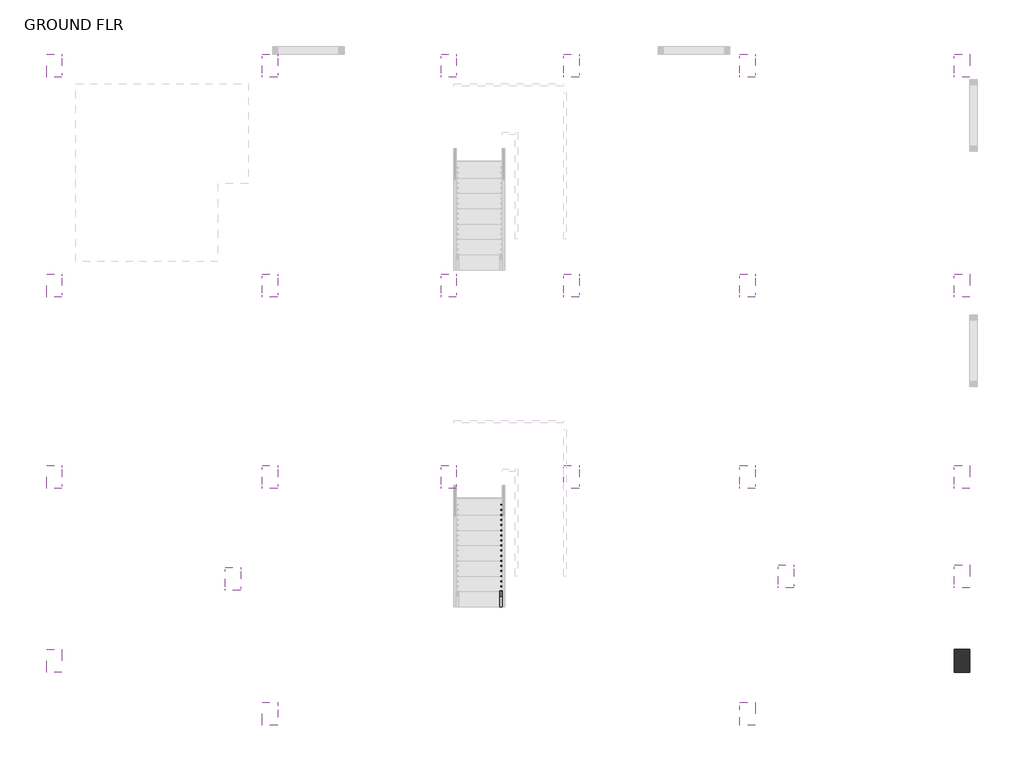
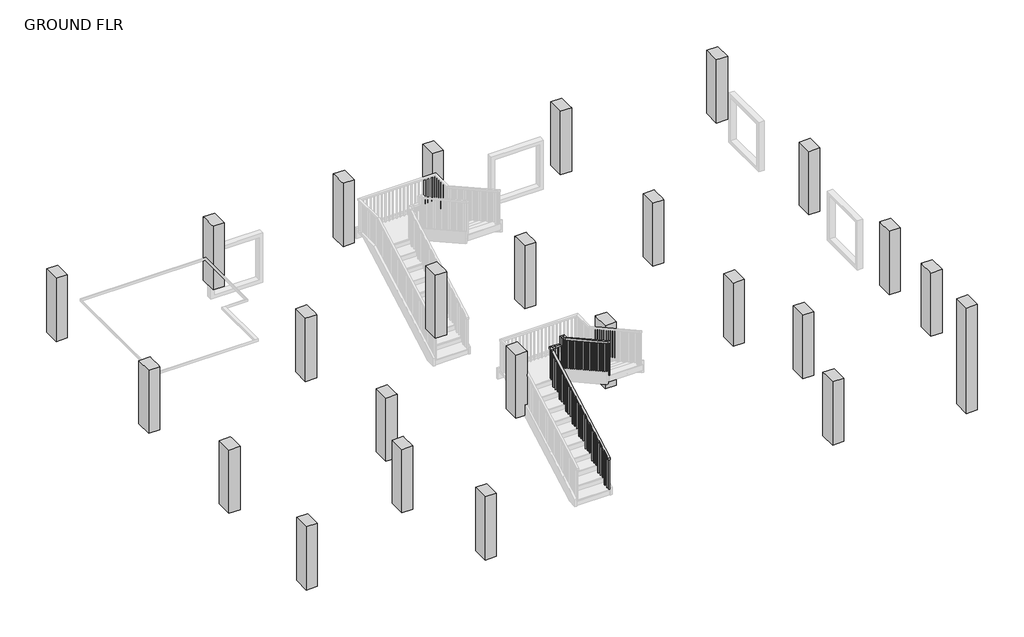
# One storey, part 1 of 4: 25 columns, 1 railing.
"""IFC4 building model written with IfcOpenShell, lengths in millimetres."""

from ifc_helpers import new_model, si_unit, frame, origin, place, context, project, spatial, polyline, outline, extrude, faceted_brep, transform, mapped, element, save
from components import column_6a931455

model = new_model("IFC4")

# Units and contexts
model_context = context("Model", 3, world=origin())
ifc_project = project(units=[si_unit("LENGTHUNIT", "METRE", prefix="MILLI")], contexts=[model_context])

# Site, building, storey
site = spatial("IfcSite", under=ifc_project)
building = spatial("IfcBuilding", under=site)
storey = spatial("IfcBuildingStorey", under=building, Name="GROUND FLR", Elevation=304.8)

# Columns
placement = place(None, origin())
element("IfcColumn", 1, ObjectType="Concrete-Rectangular-Column : 1'6\" X 1' COLUMN", at=placement, inside=storey, context=model_context, shape_type="Brep", body=[
    faceted_brep([(-8839.9786397, -1223.6061634, 1524.0), (-8839.9786397, -1680.8061634, 1524.0), (-9144.7786397, -1680.8061634, 1524.0), (-9144.7786397, -1223.6061634, 1524.0), (-8839.9786397, -1223.6061634, 3352.8), (-8839.9786397, -1299.8061634, 3352.8), (-8839.9786397, -1604.6061634, 3352.8), (-8839.9786397, -1680.8061634, 3352.8), (-8839.9786397, -1680.8061634, 2743.2), (-9144.7786397, -1680.8061634, 3352.8), (-9144.7786397, -1680.8061634, 2743.2), (-9144.7786397, -1223.6061634, 3352.8)], [[[0, 1, 2, 3]], [[4, 5, 6, 7, 8, 1, 0]], [[7, 9, 10, 2, 1, 8]], [[9, 11, 3, 2, 10]], [[11, 4, 0, 3]], [[4, 11, 9, 7, 6, 5]]]),
])
element("IfcColumn", 2, ObjectType="Concrete-Rectangular-Column : 1'6\" X 1' COLUMN", at=placement, inside=storey, context=model_context, shape_type="Brep", body=[
    faceted_brep([(-4548.1175798, -1223.6061634, 1524.0), (-4548.1175798, -1680.8061634, 1524.0), (-4852.9175798, -1680.8061634, 1524.0), (-4852.9175798, -1223.6061634, 1524.0), (-4548.1175798, -1223.6061634, 3352.8), (-4548.1175798, -1299.8061634, 3352.8), (-4548.1175798, -1604.6061634, 3352.8), (-4548.1175798, -1680.8061634, 3352.8), (-4548.1175798, -1680.8061634, 2743.2), (-4852.9175798, -1680.8061634, 3352.8), (-4852.9175798, -1680.8061634, 2743.2), (-4852.9175798, -1604.6061634, 3352.8), (-4852.9175798, -1299.8061634, 3352.8), (-4852.9175798, -1223.6061634, 3352.8)], [[[0, 1, 2, 3]], [[4, 5, 6, 7, 8, 1, 0]], [[7, 9, 10, 2, 1, 8]], [[9, 11, 12, 13, 3, 2, 10]], [[13, 4, 0, 3]], [[4, 13, 12, 11, 9, 7, 6, 5]]]),
])
element("IfcColumn", 3, ObjectType="Concrete-Rectangular-Column : 1'6\" X 1' COLUMN", at=placement, inside=storey, context=model_context, shape_type="Brep", body=[
    faceted_brep([(-992.1175798, -1223.6061634, 1524.0), (-992.1175798, -1680.8061634, 1524.0), (-1296.9175798, -1680.8061634, 1524.0), (-1296.9175798, -1223.6061634, 1524.0), (-992.1175798, -1223.6061634, 3352.8), (-992.1175798, -1299.8061634, 3352.8), (-992.1175798, -1604.6061634, 3352.8), (-992.1175798, -1680.8061634, 3352.8), (-992.1175798, -1680.8061634, 2743.2), (-1296.9175798, -1680.8061634, 3352.8), (-1296.9175798, -1680.8061634, 2743.2), (-1296.9175798, -1604.6061634, 3352.8), (-1296.9175798, -1299.8061634, 3352.8), (-1296.9175798, -1223.6061634, 3352.8)], [[[0, 1, 2, 3]], [[4, 5, 6, 7, 8, 1, 0]], [[7, 9, 10, 2, 1, 8]], [[9, 11, 12, 13, 3, 2, 10]], [[13, 4, 0, 3]], [[4, 13, 12, 11, 9, 7, 6, 5]]]),
])
element("IfcColumn", 4, ObjectType="Concrete-Rectangular-Column : 1'6\" X 1' COLUMN", at=placement, inside=storey, context=model_context, shape_type="Brep", body=[
    faceted_brep([(1446.2824202, -1223.6061634, 1524.0), (1446.2824202, -1680.8061634, 1524.0), (1141.4824202, -1680.8061634, 1524.0), (1141.4824202, -1223.6061634, 1524.0), (1446.2824202, -1223.6061634, 3352.8), (1446.2824202, -1299.8061634, 3352.8), (1446.2824202, -1604.6061634, 3352.8), (1446.2824202, -1680.8061634, 3352.8), (1446.2824202, -1680.8061634, 2743.2), (1141.4824202, -1680.8061634, 3352.8), (1141.4824202, -1680.8061634, 2743.2), (1141.4824202, -1604.6061634, 3352.8), (1141.4824202, -1299.8061634, 3352.8), (1141.4824202, -1223.6061634, 3352.8)], [[[0, 1, 2, 3]], [[4, 5, 6, 7, 8, 1, 0]], [[7, 9, 10, 2, 1, 8]], [[9, 11, 12, 13, 3, 2, 10]], [[13, 4, 0, 3]], [[4, 13, 12, 11, 9, 7, 6, 5]]]),
])
element("IfcColumn", 5, ObjectType="Concrete-Rectangular-Column : 1'6\" X 1' COLUMN", at=placement, inside=storey, context=model_context, shape_type="Brep", body=[
    faceted_brep([(4951.4824202, -1223.6061634, 1524.0), (4951.4824202, -1680.8061634, 1524.0), (4646.6824202, -1680.8061634, 1524.0), (4646.6824202, -1223.6061634, 1524.0), (4951.4824202, -1223.6061634, 3352.8), (4951.4824202, -1299.8061634, 3352.8), (4951.4824202, -1604.6061634, 3352.8), (4951.4824202, -1680.8061634, 3352.8), (4951.4824202, -1680.8061634, 2743.2), (4646.6824202, -1680.8061634, 3352.8), (4646.6824202, -1680.8061634, 2743.2), (4646.6824202, -1604.6061634, 3352.8), (4646.6824202, -1299.8061634, 3352.8), (4646.6824202, -1223.6061634, 3352.8)], [[[0, 1, 2, 3]], [[4, 5, 6, 7, 8, 1, 0]], [[7, 9, 10, 2, 1, 8]], [[9, 11, 12, 13, 3, 2, 10]], [[13, 4, 0, 3]], [[4, 13, 12, 11, 9, 7, 6, 5]]]),
])
element("IfcColumn", 6, ObjectType="Concrete-Rectangular-Column : 1'6\" X 1' COLUMN", at=placement, inside=storey, context=model_context, shape_type="Brep", body=[
    faceted_brep([(9218.6824202, -1223.6061634, 1524.0), (9218.6824202, -1680.8061634, 1524.0), (8913.8824202, -1680.8061634, 1524.0), (8913.8824202, -1223.6061634, 1524.0), (9218.6824202, -1223.6061634, 3352.8), (9218.6824202, -1680.8061634, 3352.8), (9218.6824202, -1680.8061634, 2743.2), (8913.8824202, -1680.8061634, 3352.8), (8913.8824202, -1680.8061634, 2743.2), (8913.8824202, -1604.6061634, 3352.8), (8913.8824202, -1299.8061634, 3352.8), (8913.8824202, -1223.6061634, 3352.8)], [[[0, 1, 2, 3]], [[4, 5, 6, 1, 0]], [[5, 7, 8, 2, 1, 6]], [[7, 9, 10, 11, 3, 2, 8]], [[11, 4, 0, 3]], [[4, 11, 10, 9, 7, 5]]]),
])
element("IfcColumn", 7, ObjectType="Concrete-Rectangular-Column : 1'6\" X 1' COLUMN", at=placement, inside=storey, context=model_context, shape_type="Brep", body=[
    faceted_brep([(9218.6824202, -5600.6620333, 1524.0), (9218.6824202, -6057.8620333, 1524.0), (8913.8824202, -6057.8620333, 1524.0), (8913.8824202, -5600.6620333, 1524.0), (9218.6824202, -5600.6620333, 3352.8), (9218.6824202, -6057.8620333, 3352.8), (9218.6824202, -6057.8620333, 2743.2), (9218.6824202, -5600.6620333, 2743.2), (8913.8824202, -6057.8620333, 3352.8), (8913.8824202, -6057.8620333, 2743.2), (8913.8824202, -5981.6620333, 3352.8), (8913.8824202, -5676.8620333, 3352.8), (8913.8824202, -5600.6620333, 3352.8), (8913.8824202, -5600.6620333, 2743.2)], [[[0, 1, 2, 3]], [[4, 5, 6, 1, 0, 7]], [[5, 8, 9, 2, 1, 6]], [[8, 10, 11, 12, 13, 3, 2, 9]], [[12, 4, 7, 0, 3, 13]], [[4, 12, 11, 10, 8, 5]]]),
])
element("IfcColumn", 8, ObjectType="Concrete-Rectangular-Column : 1'6\" X 1' COLUMN", at=placement, inside=storey, context=model_context, shape_type="Brep", body=[
    faceted_brep([(4951.4824202, -5600.6620333, 1524.0), (4951.4824202, -6057.8620333, 1524.0), (4646.6824202, -6057.8620333, 1524.0), (4646.6824202, -5600.6620333, 1524.0), (4951.4824202, -5600.6620333, 3352.8), (4951.4824202, -5676.8620333, 3352.8), (4951.4824202, -5981.6620333, 3352.8), (4951.4824202, -6057.8620333, 3352.8), (4951.4824202, -6057.8620333, 2743.2), (4951.4824202, -5600.6620333, 2743.2), (4646.6824202, -6057.8620333, 3352.8), (4646.6824202, -6057.8620333, 2743.2), (4646.6824202, -5981.6620333, 3352.8), (4646.6824202, -5676.8620333, 3352.8), (4646.6824202, -5600.6620333, 3352.8), (4646.6824202, -5600.6620333, 2743.2)], [[[0, 1, 2, 3]], [[4, 5, 6, 7, 8, 1, 0, 9]], [[7, 10, 11, 2, 1, 8]], [[10, 12, 13, 14, 15, 3, 2, 11]], [[14, 4, 9, 0, 3, 15]], [[4, 14, 13, 12, 10, 7, 6, 5]]]),
])
element("IfcColumn", 9, ObjectType="Concrete-Rectangular-Column : 1'6\" X 1' COLUMN", at=placement, inside=storey, context=model_context, shape_type="Brep", body=[
    faceted_brep([(1446.2824202, -5600.6620333, 1524.0), (1446.2824202, -6057.8620333, 1524.0), (1141.4824202, -6057.8620333, 1524.0), (1141.4824202, -5600.6620333, 1524.0), (1446.2824202, -5600.6620333, 3352.8), (1446.2824202, -5676.8620333, 3352.8), (1446.2824202, -5981.6620333, 3352.8), (1446.2824202, -6057.8620333, 3352.8), (1446.2824202, -6057.8620333, 2743.2), (1446.2824202, -5600.6620333, 2743.2), (1141.4824202, -6057.8620333, 3352.8), (1141.4824202, -6057.8620333, 2743.2), (1141.4824202, -5981.6620333, 3352.8), (1141.4824202, -5676.8620333, 3352.8), (1141.4824202, -5600.6620333, 3352.8), (1141.4824202, -5600.6620333, 2743.2)], [[[0, 1, 2, 3]], [[4, 5, 6, 7, 8, 1, 0, 9]], [[7, 10, 11, 2, 1, 8]], [[10, 12, 13, 14, 15, 3, 2, 11]], [[14, 4, 9, 0, 3, 15]], [[4, 14, 13, 12, 10, 7, 6, 5]]]),
])
element("IfcColumn", 10, ObjectType="Concrete-Rectangular-Column : 1'6\" X 1' COLUMN", at=placement, inside=storey, context=model_context, shape_type="Brep", body=[
    faceted_brep([(-992.1175798, -5600.6620333, 1524.0), (-992.1175798, -6057.8620333, 1524.0), (-1296.9175798, -6057.8620333, 1524.0), (-1296.9175798, -5600.6620333, 1524.0), (-992.1175798, -5600.6620333, 3352.8), (-992.1175798, -5676.8620333, 3352.8), (-992.1175798, -5981.6620333, 3352.8), (-992.1175798, -6057.8620333, 3352.8), (-992.1175798, -6057.8620333, 2743.2), (-992.1175798, -5600.6620333, 2743.2), (-1296.9175798, -6057.8620333, 3352.8), (-1296.9175798, -6057.8620333, 2743.2), (-1296.9175798, -5981.6620333, 3352.8), (-1296.9175798, -5676.8620333, 3352.8), (-1296.9175798, -5600.6620333, 3352.8), (-1296.9175798, -5600.6620333, 2743.2)], [[[0, 1, 2, 3]], [[4, 5, 6, 7, 8, 1, 0, 9]], [[7, 10, 11, 2, 1, 8]], [[10, 12, 13, 14, 15, 3, 2, 11]], [[14, 4, 9, 0, 3, 15]], [[4, 14, 13, 12, 10, 7, 6, 5]]]),
])
element("IfcColumn", 11, ObjectType="Concrete-Rectangular-Column : 1'6\" X 1' COLUMN", at=placement, inside=storey, context=model_context, shape_type="Brep", body=[
    faceted_brep([(-4548.1175798, -5600.6620333, 1524.0), (-4548.1175798, -6057.8620333, 1524.0), (-4852.9175798, -6057.8620333, 1524.0), (-4852.9175798, -5600.6620333, 1524.0), (-4548.1175798, -5600.6620333, 3352.8), (-4548.1175798, -5676.8620333, 3352.8), (-4548.1175798, -5981.6620333, 3352.8), (-4548.1175798, -6057.8620333, 3352.8), (-4548.1175798, -6057.8620333, 2743.2), (-4548.1175798, -5600.6620333, 2743.2), (-4852.9175798, -6057.8620333, 3352.8), (-4852.9175798, -6057.8620333, 2743.2), (-4852.9175798, -5981.6620333, 3352.8), (-4852.9175798, -5676.8620333, 3352.8), (-4852.9175798, -5600.6620333, 3352.8), (-4852.9175798, -5600.6620333, 2743.2)], [[[0, 1, 2, 3]], [[4, 5, 6, 7, 8, 1, 0, 9]], [[7, 10, 11, 2, 1, 8]], [[10, 12, 13, 14, 15, 3, 2, 11]], [[14, 4, 9, 0, 3, 15]], [[4, 14, 13, 12, 10, 7, 6, 5]]]),
])
element("IfcColumn", 12, ObjectType="Concrete-Rectangular-Column : 1'6\" X 1' COLUMN", at=placement, inside=storey, context=model_context, shape_type="Brep", body=[
    faceted_brep([(-8839.9786397, -5600.6620333, 1524.0), (-8839.9786397, -6057.8620333, 1524.0), (-9144.7786397, -6057.8620333, 1524.0), (-9144.7786397, -5600.6620333, 1524.0), (-8839.9786397, -5600.6620333, 3352.8), (-8839.9786397, -5676.8620333, 3352.8), (-8839.9786397, -5981.6620333, 3352.8), (-8839.9786397, -6057.8620333, 3352.8), (-8839.9786397, -6057.8620333, 2743.2), (-8839.9786397, -5600.6620333, 2743.2), (-9144.7786397, -6057.8620333, 3352.8), (-9144.7786397, -6057.8620333, 2743.2), (-9144.7786397, -5600.6620333, 3352.8), (-9144.7786397, -5600.6620333, 2743.2)], [[[0, 1, 2, 3]], [[4, 5, 6, 7, 8, 1, 0, 9]], [[7, 10, 11, 2, 1, 8]], [[10, 12, 13, 3, 2, 11]], [[12, 4, 9, 0, 3, 13]], [[4, 12, 10, 7, 6, 5]]]),
])
element("IfcColumn", 13, ObjectType="Concrete-Rectangular-Column : 1'6\" X 1' COLUMN", at=placement, inside=storey, context=model_context, shape_type="Brep", body=[
    faceted_brep([(-8839.9786397, -9410.6620333, 1524.0), (-8839.9786397, -9867.8620333, 1524.0), (-9144.7786397, -9867.8620333, 1524.0), (-9144.7786397, -9410.6620333, 1524.0), (-8839.9786397, -9410.6620333, 3352.8), (-8839.9786397, -9486.8620333, 3352.8), (-8839.9786397, -9791.6620333, 3352.8), (-8839.9786397, -9867.8620333, 3352.8), (-8839.9786397, -9867.8620333, 2743.2), (-8839.9786397, -9410.6620333, 2743.2), (-9144.7786397, -9867.8620333, 3352.8), (-9144.7786397, -9867.8620333, 2743.2), (-9144.7786397, -9410.6620333, 3352.8), (-9144.7786397, -9410.6620333, 2743.2)], [[[0, 1, 2, 3]], [[4, 5, 6, 7, 8, 1, 0, 9]], [[7, 10, 11, 2, 1, 8]], [[10, 12, 13, 3, 2, 11]], [[12, 4, 9, 0, 3, 13]], [[4, 12, 10, 7, 6, 5]]]),
])
element("IfcColumn", 14, ObjectType="Concrete-Rectangular-Column : 1'6\" X 1' COLUMN", at=placement, inside=storey, context=model_context, shape_type="Brep", body=[
    faceted_brep([(-4548.1175798, -9410.6620333, 1524.0), (-4548.1175798, -9867.8620333, 1524.0), (-4852.9175798, -9867.8620333, 1524.0), (-4852.9175798, -9410.6620333, 1524.0), (-4548.1175798, -9410.6620333, 3352.8), (-4548.1175798, -9486.8620333, 3352.8), (-4548.1175798, -9791.6620333, 3352.8), (-4548.1175798, -9867.8620333, 3352.8), (-4548.1175798, -9867.8620333, 2743.2), (-4548.1175798, -9410.6620333, 2743.2), (-4852.9175798, -9867.8620333, 3352.8), (-4852.9175798, -9867.8620333, 2743.2), (-4852.9175798, -9791.6620333, 3352.8), (-4852.9175798, -9486.8620333, 3352.8), (-4852.9175798, -9410.6620333, 3352.8), (-4852.9175798, -9410.6620333, 2743.2)], [[[0, 1, 2, 3]], [[4, 5, 6, 7, 8, 1, 0, 9]], [[7, 10, 11, 2, 1, 8]], [[10, 12, 13, 14, 15, 3, 2, 11]], [[14, 4, 9, 0, 3, 15]], [[4, 14, 13, 12, 10, 7, 6, 5]]]),
])
element("IfcColumn", 15, ObjectType="Concrete-Rectangular-Column : 1'6\" X 1' COLUMN", at=placement, inside=storey, context=model_context, shape_type="Brep", body=[
    faceted_brep([(-992.1175798, -9410.6620333, 1524.0), (-992.1175798, -9867.8620333, 1524.0), (-1296.9175798, -9867.8620333, 1524.0), (-1296.9175798, -9410.6620333, 1524.0), (-992.1175798, -9410.6620333, 3352.8), (-992.1175798, -9486.8620333, 3352.8), (-992.1175798, -9791.6620333, 3352.8), (-992.1175798, -9867.8620333, 3352.8), (-992.1175798, -9410.6620333, 2743.2), (-1296.9175798, -9867.8620333, 3352.8), (-1296.9175798, -9791.6620333, 3352.8), (-1296.9175798, -9486.8620333, 3352.8), (-1296.9175798, -9410.6620333, 3352.8), (-1296.9175798, -9410.6620333, 2743.2)], [[[0, 1, 2, 3]], [[4, 5, 6, 7, 1, 0, 8]], [[7, 9, 2, 1]], [[9, 10, 11, 12, 13, 3, 2]], [[12, 4, 8, 0, 3, 13]], [[4, 12, 11, 10, 9, 7, 6, 5]]]),
])
element("IfcColumn", 16, ObjectType="Concrete-Rectangular-Column : 1'6\" X 1' COLUMN", at=placement, inside=storey, context=model_context, shape_type="Brep", body=[
    faceted_brep([(9218.6824202, -11391.8620333, 1524.0), (9218.6824202, -11849.0620333, 1524.0), (8913.8824202, -11849.0620333, 1524.0), (8913.8824202, -11391.8620333, 1524.0), (9218.6824202, -11391.8620333, 3352.8), (9218.6824202, -11849.0620333, 3352.8), (9218.6824202, -11391.8620333, 2743.2), (8913.8824202, -11849.0620333, 3352.8), (8913.8824202, -11772.8620333, 3352.8), (8913.8824202, -11468.0620333, 3352.8), (8913.8824202, -11391.8620333, 3352.8), (8913.8824202, -11391.8620333, 2743.2)], [[[0, 1, 2, 3]], [[4, 5, 1, 0, 6]], [[5, 7, 2, 1]], [[7, 8, 9, 10, 11, 3, 2]], [[10, 4, 6, 0, 3, 11]], [[4, 10, 9, 8, 7, 5]]]),
])
element("IfcColumn", 17, ObjectType="Concrete-Rectangular-Column : 1'6\" X 1' COLUMN", at=placement, inside=storey, context=model_context, shape_type="Brep", body=[
    faceted_brep([(9218.6824202, -9410.6620333, 1524.0), (9218.6824202, -9867.8620333, 1524.0), (8913.8824202, -9867.8620333, 1524.0), (8913.8824202, -9410.6620333, 1524.0), (9218.6824202, -9410.6620333, 3352.8), (9218.6824202, -9867.8620333, 3352.8), (9218.6824202, -9867.8620333, 2743.2), (9218.6824202, -9410.6620333, 2743.2), (8913.8824202, -9867.8620333, 3352.8), (8913.8824202, -9867.8620333, 2743.2), (8913.8824202, -9791.6620333, 3352.8), (8913.8824202, -9486.8620333, 3352.8), (8913.8824202, -9410.6620333, 3352.8), (8913.8824202, -9410.6620333, 2743.2)], [[[0, 1, 2, 3]], [[4, 5, 6, 1, 0, 7]], [[5, 8, 9, 2, 1, 6]], [[8, 10, 11, 12, 13, 3, 2, 9]], [[12, 4, 7, 0, 3, 13]], [[4, 12, 11, 10, 8, 5]]]),
])
element("IfcColumn", 18, ObjectType="Concrete-Rectangular-Column : 1'6\" X 1' COLUMN", at=placement, inside=storey, context=model_context, shape_type="Brep", body=[
    faceted_brep([(4951.4824202, -9410.6620333, 1524.0), (4951.4824202, -9867.8620333, 1524.0), (4646.6824202, -9867.8620333, 1524.0), (4646.6824202, -9410.6620333, 1524.0), (4951.4824202, -9410.6620333, 3352.8), (4951.4824202, -9486.8620333, 3352.8), (4951.4824202, -9791.6620333, 3352.8), (4951.4824202, -9867.8620333, 3352.8), (4951.4824202, -9867.8620333, 2743.2), (4951.4824202, -9410.6620333, 2743.2), (4646.6824202, -9867.8620333, 3352.8), (4646.6824202, -9867.8620333, 2743.2), (4646.6824202, -9791.6620333, 3352.8), (4646.6824202, -9486.8620333, 3352.8), (4646.6824202, -9410.6620333, 3352.8), (4646.6824202, -9410.6620333, 2743.2)], [[[0, 1, 2, 3]], [[4, 5, 6, 7, 8, 1, 0, 9]], [[7, 10, 11, 2, 1, 8]], [[10, 12, 13, 14, 15, 3, 2, 11]], [[14, 4, 9, 0, 3, 15]], [[4, 14, 13, 12, 10, 7, 6, 5]]]),
])
element("IfcColumn", 19, ObjectType="Concrete-Rectangular-Column : 1'6\" X 1' COLUMN", at=placement, inside=storey, context=model_context, shape_type="Brep", body=[
    faceted_brep([(1446.2824202, -9410.6620333, 1524.0), (1446.2824202, -9867.8620333, 1524.0), (1141.4824202, -9867.8620333, 1524.0), (1141.4824202, -9410.6620333, 1524.0), (1446.2824202, -9410.6620333, 3352.8), (1446.2824202, -9486.8620333, 3352.8), (1446.2824202, -9791.6620333, 3352.8), (1446.2824202, -9867.8620333, 3352.8), (1446.2824202, -9410.6620333, 2743.2), (1141.4824202, -9867.8620333, 3352.8), (1141.4824202, -9791.6620333, 3352.8), (1141.4824202, -9486.8620333, 3352.8), (1141.4824202, -9410.6620333, 3352.8), (1141.4824202, -9410.6620333, 2743.2)], [[[0, 1, 2, 3]], [[4, 5, 6, 7, 1, 0, 8]], [[7, 9, 2, 1]], [[9, 10, 11, 12, 13, 3, 2]], [[12, 4, 8, 0, 3, 13]], [[4, 12, 11, 10, 9, 7, 6, 5]]]),
])
element("IfcColumn", 20, ObjectType="Concrete-Rectangular-Column : 1'6\" X 1' COLUMN", at=placement, inside=storey, context=model_context, shape_type="Brep", body=[
    faceted_brep([(-4548.1175798, -14119.6402089, 1524.0), (-4548.1175798, -14576.8402089, 1524.0), (-4852.9175798, -14576.8402089, 1524.0), (-4852.9175798, -14119.6402089, 1524.0), (-4548.1175798, -14119.6402089, 3352.8), (-4548.1175798, -14272.0402089, 3352.8), (-4548.1175798, -14576.8402089, 3352.8), (-4548.1175798, -14576.8402089, 2743.2), (-4548.1175798, -14119.6402089, 2743.2), (-4852.9175798, -14576.8402089, 3352.8), (-4852.9175798, -14119.6402089, 3352.8), (-4852.9175798, -14119.6402089, 2743.2)], [[[0, 1, 2, 3]], [[4, 5, 6, 7, 1, 0, 8]], [[6, 9, 2, 1, 7]], [[9, 10, 11, 3, 2]], [[10, 4, 8, 0, 3, 11]], [[4, 10, 9, 6, 5]]]),
])
element("IfcColumn", 21, ObjectType="Concrete-Rectangular-Column : 1'6\" X 1' COLUMN", at=placement, inside=storey, context=model_context, shape_type="Brep", body=[
    faceted_brep([(-8839.9786397, -13068.2620333, 1524.0), (-8839.9786397, -13525.4620333, 1524.0), (-9144.7786397, -13525.4620333, 1524.0), (-9144.7786397, -13068.2620333, 1524.0), (-8839.9786397, -13068.2620333, 3352.8), (-8839.9786397, -13525.4620333, 3352.8), (-8839.9786397, -13068.2620333, 2743.2), (-9144.7786397, -13525.4620333, 3352.8), (-9144.7786397, -13068.2620333, 3352.8), (-9144.7786397, -13068.2620333, 2743.2)], [[[0, 1, 2, 3]], [[4, 5, 1, 0, 6]], [[5, 7, 2, 1]], [[7, 8, 9, 3, 2]], [[8, 4, 6, 0, 3, 9]], [[4, 8, 7, 5]]]),
])
element("IfcColumn", 22, ObjectType="Concrete-Rectangular-Column : 1'6\" X 1' COLUMN", at=placement, inside=storey, context=model_context, shape_type="Brep", body=[
    faceted_brep([(-5284.7175798, -11442.6620333, 1524.0), (-5284.7175798, -11899.8620333, 1524.0), (-5589.5175798, -11899.8620333, 1524.0), (-5589.5175798, -11442.6620333, 1524.0), (-5284.7175798, -11442.6620333, 3352.8), (-5284.7175798, -11518.8620333, 3352.8), (-5284.7175798, -11823.6620333, 3352.8), (-5284.7175798, -11899.8620333, 3352.8), (-5589.5175798, -11899.8620333, 3352.8), (-5589.5175798, -11823.6620333, 3352.8), (-5589.5175798, -11518.8620333, 3352.8), (-5589.5175798, -11442.6620333, 3352.8)], [[[0, 1, 2, 3]], [[4, 5, 6, 7, 1, 0]], [[7, 8, 2, 1]], [[8, 9, 10, 11, 3, 2]], [[11, 4, 0, 3]], [[4, 11, 10, 9, 8, 7, 6, 5]]]),
])
element("IfcColumn", 23, ObjectType="Concrete-Rectangular-Column : 1'6\" X 1' COLUMN", at=placement, inside=storey, context=model_context, shape_type="Brep", body=[
    faceted_brep([(5713.4824202, -11391.8620333, 1524.0), (5713.4824202, -11849.0620333, 1524.0), (5408.6824202, -11849.0620333, 1524.0), (5408.6824202, -11391.8620333, 1524.0), (5713.4824202, -11391.8620333, 3352.8), (5713.4824202, -11468.0620333, 3352.8), (5713.4824202, -11772.8620333, 3352.8), (5713.4824202, -11849.0620333, 3352.8), (5408.6824202, -11849.0620333, 3352.8), (5408.6824202, -11772.8620333, 3352.8), (5408.6824202, -11468.0620333, 3352.8), (5408.6824202, -11391.8620333, 3352.8)], [[[0, 1, 2, 3]], [[4, 5, 6, 7, 1, 0]], [[7, 8, 2, 1]], [[8, 9, 10, 11, 3, 2]], [[11, 4, 0, 3]], [[4, 11, 10, 9, 8, 7, 6, 5]]]),
])
element("IfcColumn", 24, ObjectType="Concrete-Rectangular-Column : 1'6\" X 1' COLUMN", at=placement, inside=storey, context=model_context, shape_type="Brep", body=[
    faceted_brep([(4951.4824202, -14119.6402089, 1524.0), (4951.4824202, -14576.8402089, 1524.0), (4646.6824202, -14576.8402089, 1524.0), (4646.6824202, -14119.6402089, 1524.0), (4951.4824202, -14119.6402089, 3352.8), (4951.4824202, -14576.8402089, 3352.8), (4951.4824202, -14119.6402089, 2743.2), (4646.6824202, -14576.8402089, 3352.8), (4646.6824202, -14576.8402089, 2743.2), (4646.6824202, -14272.0402089, 3352.8), (4646.6824202, -14119.6402089, 3352.8), (4646.6824202, -14119.6402089, 2743.2)], [[[0, 1, 2, 3]], [[4, 5, 1, 0, 6]], [[5, 7, 8, 2, 1]], [[7, 9, 10, 11, 3, 2, 8]], [[10, 4, 6, 0, 3, 11]], [[4, 10, 9, 7, 5]]]),
])
column_shape = column_6a931455(model_context)
element("IfcColumn", 25, ObjectType="Concrete-Rectangular-Column : 1'6\" X 1' COLUMN", at=placement, inside=storey, context=model_context, shape_type="MappedRepresentation", body=[
    mapped(column_shape, transform((9066.2824202, -13294.1402089, 0.0), x_axis=(1.0, 0.0, 0.0), y_axis=(0.0, 1.0, 0.0), z_axis=(0.0, 0.0, 1.0))),
])

# Railing
element("IfcRailing", 26, ObjectType="Handrail - Rectangular", at=placement, inside=storey, context=model_context, shape_type="SolidModel", body=[
    faceted_brep([(-128.5175798, -12221.8061634, 1388.5333333), (-128.5175798, -12221.8061634, 1330.420221), (-77.7175798, -12221.8061634, 1330.420221), (-77.7175798, -12221.8061634, 1388.5333333), (-128.5175798, -9554.8061634, 2870.2), (-128.5175798, -9504.0061634, 2840.3091099), (-77.7175798, -9504.0061634, 2840.3091099), (-77.7175798, -9554.8061634, 2870.2), (-128.5175798, -9554.8061634, 2912.5333333), (-128.5175798, -9504.0061634, 2861.7333333), (-77.7175798, -9504.0061634, 2861.7333333), (-77.7175798, -9554.8061634, 2912.5333333), (-128.5175798, -9427.8061634, 2912.5333333), (-128.5175798, -9427.8061634, 2861.7333333), (-77.7175798, -9478.6061634, 2861.7333333), (-77.7175798, -9478.6061634, 2912.5333333), (-1.5175798, -9427.8061634, 2912.5333333), (-1.5175798, -9427.8061634, 2861.7333333), (-1.5175798, -9478.6061634, 2861.7333333), (-1.5175798, -9478.6061634, 2912.5333333), (150.8824202, -9427.8061634, 2912.5333333), (201.6824202, -9427.8061634, 2861.7333333), (201.6824202, -9478.6061634, 2861.7333333), (150.8824202, -9478.6061634, 2912.5333333), (150.8824202, -9427.8061634, 3124.2), (201.6824202, -9427.8061634, 3073.4), (201.6824202, -9478.6061634, 3073.4), (150.8824202, -9478.6061634, 3124.2), (277.8824202, -9427.8061634, 3124.2), (277.8824202, -9427.8061634, 3073.4), (227.0824202, -9478.6061634, 3073.4), (227.0824202, -9478.6061634, 3124.2), (277.8824202, -9554.8061634, 3124.2), (277.8824202, -9567.9697656, 3073.4), (227.0824202, -9567.9697656, 3073.4), (227.0824202, -9554.8061634, 3124.2), (277.8824202, -11612.2061634, 4267.2), (227.0824202, -11612.2061634, 4267.2), (227.0824202, -11612.2061634, 4209.0868876), (277.8824202, -11612.2061634, 4209.0868876)], [[[0, 1, 2, 3]], [[1, 0, 4, 5]], [[2, 1, 5, 6]], [[3, 2, 6, 7]], [[0, 3, 7, 4]], [[5, 4, 8, 9]], [[6, 5, 9, 10]], [[7, 6, 10, 11]], [[4, 7, 11, 8]], [[9, 8, 12, 13]], [[10, 9, 13, 14]], [[11, 10, 14, 15]], [[8, 11, 15, 12]], [[13, 12, 16, 17]], [[14, 13, 17, 18]], [[15, 14, 18, 19]], [[12, 15, 19, 16]], [[17, 16, 20, 21]], [[18, 17, 21, 22]], [[19, 18, 22, 23]], [[16, 19, 23, 20]], [[21, 20, 24, 25]], [[22, 21, 25, 26]], [[23, 22, 26, 27]], [[20, 23, 27, 24]], [[25, 24, 28, 29]], [[26, 25, 29, 30]], [[27, 26, 30, 31]], [[24, 27, 31, 28]], [[29, 28, 32, 33]], [[30, 29, 33, 34]], [[31, 30, 34, 35]], [[28, 31, 35, 32]], [[36, 37, 38, 39]], [[33, 32, 36, 39]], [[34, 33, 39, 38]], [[35, 34, 38, 37]], [[32, 35, 37, 36]]]),
    extrude(outline(polyline([(-11596.3311634, 4200.2674432), (-11577.2811634, 4189.6841099), (-11577.2811634, 3183.4666667), (-11596.3311634, 3183.4666667), (-11596.3311634, 4200.2674432)])), frame((242.9574202, 0.0, 0.0), z_axis=(1.0, 0.0, 0.0), x_axis=(0.0, 1.0, 0.0)), (0.0, 0.0, 1.0), 19.05),
    extrude(outline(polyline([(-11494.7311634, 4143.8229988), (-11475.6811634, 4133.2396654), (-11475.6811634, 3183.4666667), (-11494.7311634, 3183.4666667), (-11494.7311634, 4143.8229988)])), frame((242.9574202, 0.0, 0.0), z_axis=(1.0, 0.0, 0.0), x_axis=(0.0, 1.0, 0.0)), (0.0, 0.0, 1.0), 19.05),
    extrude(outline(polyline([(-11393.1311634, 4087.3785543), (-11374.0811634, 4076.795221), (-11374.0811634, 3183.4666667), (-11393.1311634, 3183.4666667), (-11393.1311634, 4087.3785543)])), frame((242.9574202, 0.0, 0.0), z_axis=(1.0, 0.0, 0.0), x_axis=(0.0, 1.0, 0.0)), (0.0, 0.0, 1.0), 19.05),
    extrude(outline(polyline([(-11291.5311634, 4030.9341099), (-11272.4811634, 4020.3507765), (-11272.4811634, 3014.1333333), (-11291.5311634, 3014.1333333), (-11291.5311634, 4030.9341099)])), frame((242.9574202, 0.0, 0.0), z_axis=(1.0, 0.0, 0.0), x_axis=(0.0, 1.0, 0.0)), (0.0, 0.0, 1.0), 19.05),
    extrude(outline(polyline([(-11189.9311634, 3974.4896654), (-11170.8811634, 3963.9063321), (-11170.8811634, 3014.1333333), (-11189.9311634, 3014.1333333), (-11189.9311634, 3974.4896654)])), frame((242.9574202, 0.0, 0.0), z_axis=(1.0, 0.0, 0.0), x_axis=(0.0, 1.0, 0.0)), (0.0, 0.0, 1.0), 19.05),
    extrude(outline(polyline([(-11088.3311634, 3918.045221), (-11069.2811634, 3907.4618876), (-11069.2811634, 3014.1333333), (-11088.3311634, 3014.1333333), (-11088.3311634, 3918.045221)])), frame((242.9574202, 0.0, 0.0), z_axis=(1.0, 0.0, 0.0), x_axis=(0.0, 1.0, 0.0)), (0.0, 0.0, 1.0), 19.05),
    extrude(outline(polyline([(-10986.7311634, 3861.6007765), (-10967.6811634, 3851.0174432), (-10967.6811634, 2844.8), (-10986.7311634, 2844.8), (-10986.7311634, 3861.6007765)])), frame((242.9574202, 0.0, 0.0), z_axis=(1.0, 0.0, 0.0), x_axis=(0.0, 1.0, 0.0)), (0.0, 0.0, 1.0), 19.05),
    extrude(outline(polyline([(-10885.1311634, 3805.1563321), (-10866.0811634, 3794.5729988), (-10866.0811634, 2844.8), (-10885.1311634, 2844.8), (-10885.1311634, 3805.1563321)])), frame((242.9574202, 0.0, 0.0), z_axis=(1.0, 0.0, 0.0), x_axis=(0.0, 1.0, 0.0)), (0.0, 0.0, 1.0), 19.05),
    extrude(outline(polyline([(-10783.5311634, 3748.7118876), (-10764.4811634, 3738.1285543), (-10764.4811634, 2844.8), (-10783.5311634, 2844.8), (-10783.5311634, 3748.7118876)])), frame((242.9574202, 0.0, 0.0), z_axis=(1.0, 0.0, 0.0), x_axis=(0.0, 1.0, 0.0)), (0.0, 0.0, 1.0), 19.05),
    extrude(outline(polyline([(-10681.9311634, 3692.2674432), (-10662.8811634, 3681.6841099), (-10662.8811634, 2675.4666667), (-10681.9311634, 2675.4666667), (-10681.9311634, 3692.2674432)])), frame((242.9574202, 0.0, 0.0), z_axis=(1.0, 0.0, 0.0), x_axis=(0.0, 1.0, 0.0)), (0.0, 0.0, 1.0), 19.05),
    extrude(outline(polyline([(-10580.3311634, 3635.8229988), (-10561.2811634, 3625.2396654), (-10561.2811634, 2675.4666667), (-10580.3311634, 2675.4666667), (-10580.3311634, 3635.8229988)])), frame((242.9574202, 0.0, 0.0), z_axis=(1.0, 0.0, 0.0), x_axis=(0.0, 1.0, 0.0)), (0.0, 0.0, 1.0), 19.05),
    extrude(outline(polyline([(-10478.7311634, 3579.3785543), (-10459.6811634, 3568.795221), (-10459.6811634, 2675.4666667), (-10478.7311634, 2675.4666667), (-10478.7311634, 3579.3785543)])), frame((242.9574202, 0.0, 0.0), z_axis=(1.0, 0.0, 0.0), x_axis=(0.0, 1.0, 0.0)), (0.0, 0.0, 1.0), 19.05),
    extrude(outline(polyline([(-10377.1311634, 3522.9341099), (-10358.0811634, 3512.3507765), (-10358.0811634, 2506.1333333), (-10377.1311634, 2506.1333333), (-10377.1311634, 3522.9341099)])), frame((242.9574202, 0.0, 0.0), z_axis=(1.0, 0.0, 0.0), x_axis=(0.0, 1.0, 0.0)), (0.0, 0.0, 1.0), 19.05),
    extrude(outline(polyline([(-10275.5311634, 3466.4896654), (-10256.4811634, 3455.9063321), (-10256.4811634, 2506.1333333), (-10275.5311634, 2506.1333333), (-10275.5311634, 3466.4896654)])), frame((242.9574202, 0.0, 0.0), z_axis=(1.0, 0.0, 0.0), x_axis=(0.0, 1.0, 0.0)), (0.0, 0.0, 1.0), 19.05),
    extrude(outline(polyline([(-10173.9311634, 3410.045221), (-10154.8811634, 3399.4618876), (-10154.8811634, 2506.1333333), (-10173.9311634, 2506.1333333), (-10173.9311634, 3410.045221)])), frame((242.9574202, 0.0, 0.0), z_axis=(1.0, 0.0, 0.0), x_axis=(0.0, 1.0, 0.0)), (0.0, 0.0, 1.0), 19.05),
    extrude(outline(polyline([(-10072.3311634, 3353.6007765), (-10053.2811634, 3343.0174432), (-10053.2811634, 2336.8), (-10072.3311634, 2336.8), (-10072.3311634, 3353.6007765)])), frame((242.9574202, 0.0, 0.0), z_axis=(1.0, 0.0, 0.0), x_axis=(0.0, 1.0, 0.0)), (0.0, 0.0, 1.0), 19.05),
    extrude(outline(polyline([(-9970.7311634, 3297.1563321), (-9951.6811634, 3286.5729988), (-9951.6811634, 2336.8), (-9970.7311634, 2336.8), (-9970.7311634, 3297.1563321)])), frame((242.9574202, 0.0, 0.0), z_axis=(1.0, 0.0, 0.0), x_axis=(0.0, 1.0, 0.0)), (0.0, 0.0, 1.0), 19.05),
    extrude(outline(polyline([(-9869.1311634, 3240.7118876), (-9850.0811634, 3230.1285543), (-9850.0811634, 2336.8), (-9869.1311634, 2336.8), (-9869.1311634, 3240.7118876)])), frame((242.9574202, 0.0, 0.0), z_axis=(1.0, 0.0, 0.0), x_axis=(0.0, 1.0, 0.0)), (0.0, 0.0, 1.0), 19.05),
    extrude(outline(polyline([(-9767.5311634, 3184.2674432), (-9748.4811634, 3173.6841099), (-9748.4811634, 2167.4666667), (-9767.5311634, 2167.4666667), (-9767.5311634, 3184.2674432)])), frame((242.9574202, 0.0, 0.0), z_axis=(1.0, 0.0, 0.0), x_axis=(0.0, 1.0, 0.0)), (0.0, 0.0, 1.0), 19.05),
    extrude(outline(polyline([(-9665.9311634, 3127.8229988), (-9646.8811634, 3117.2396654), (-9646.8811634, 2167.4666667), (-9665.9311634, 2167.4666667), (-9665.9311634, 3127.8229988)])), frame((242.9574202, 0.0, 0.0), z_axis=(1.0, 0.0, 0.0), x_axis=(0.0, 1.0, 0.0)), (0.0, 0.0, 1.0), 19.05),
    extrude(outline(polyline([(-9564.3311634, 3071.3785543), (-9545.2811634, 3060.795221), (-9545.2811634, 2167.4666667), (-9564.3311634, 2167.4666667), (-9564.3311634, 3071.3785543)])), frame((242.9574202, 0.0, 0.0), z_axis=(1.0, 0.0, 0.0), x_axis=(0.0, 1.0, 0.0)), (0.0, 0.0, 1.0), 19.05),
    extrude(outline(polyline([(192.1574202, -9462.7311634), (192.1574202, -9443.6811634), (211.2074202, -9443.6811634), (211.2074202, -9462.7311634), (192.1574202, -9462.7311634)])), frame((0.0, 0.0, 1998.1333333), z_axis=(0.0, 0.0, 1.0), x_axis=(1.0, 0.0, 0.0)), (0.0, 0.0, 1.0), 1075.2666667),
    extrude(outline(polyline([(90.5574202, -9462.7311634), (90.5574202, -9443.6811634), (109.6074202, -9443.6811634), (109.6074202, -9462.7311634), (90.5574202, -9462.7311634)])), frame((0.0, 0.0, 1998.1333333), z_axis=(0.0, 0.0, 1.0), x_axis=(1.0, 0.0, 0.0)), (0.0, 0.0, 1.0), 863.6),
    extrude(outline(polyline([(-11.0425798, -9462.7311634), (-11.0425798, -9443.6811634), (8.0074202, -9443.6811634), (8.0074202, -9462.7311634), (-11.0425798, -9462.7311634)])), frame((0.0, 0.0, 1998.1333333), z_axis=(0.0, 0.0, 1.0), x_axis=(1.0, 0.0, 0.0)), (0.0, 0.0, 1.0), 863.6),
    extrude(outline(polyline([(-93.5925798, -9488.1311634), (-112.6425798, -9488.1311634), (-112.6425798, -9469.0811634), (-93.5925798, -9469.0811634), (-93.5925798, -9488.1311634)])), frame((0.0, 0.0, 1998.1333333), z_axis=(0.0, 0.0, 1.0), x_axis=(1.0, 0.0, 0.0)), (0.0, 0.0, 1.0), 863.6),
    extrude(outline(polyline([(-9589.7311634, 2792.6841099), (-9570.6811634, 2803.2674432), (-9570.6811634, 1828.8), (-9589.7311634, 1828.8), (-9589.7311634, 2792.6841099)])), frame((-112.6425798, 0.0, 0.0), z_axis=(1.0, 0.0, 0.0), x_axis=(0.0, 1.0, 0.0)), (0.0, 0.0, 1.0), 19.05),
    extrude(outline(polyline([(-9691.3311634, 2736.2396654), (-9672.2811634, 2746.8229988), (-9672.2811634, 1828.8), (-9691.3311634, 1828.8), (-9691.3311634, 2736.2396654)])), frame((-112.6425798, 0.0, 0.0), z_axis=(1.0, 0.0, 0.0), x_axis=(0.0, 1.0, 0.0)), (0.0, 0.0, 1.0), 19.05),
    extrude(outline(polyline([(-9792.9311634, 2679.795221), (-9773.8811634, 2690.3785543), (-9773.8811634, 1828.8), (-9792.9311634, 1828.8), (-9792.9311634, 2679.795221)])), frame((-112.6425798, 0.0, 0.0), z_axis=(1.0, 0.0, 0.0), x_axis=(0.0, 1.0, 0.0)), (0.0, 0.0, 1.0), 19.05),
    extrude(outline(polyline([(-9894.5311634, 2623.3507765), (-9875.4811634, 2633.9341099), (-9875.4811634, 1659.4666667), (-9894.5311634, 1659.4666667), (-9894.5311634, 2623.3507765)])), frame((-112.6425798, 0.0, 0.0), z_axis=(1.0, 0.0, 0.0), x_axis=(0.0, 1.0, 0.0)), (0.0, 0.0, 1.0), 19.05),
    extrude(outline(polyline([(-9996.1311634, 2566.9063321), (-9977.0811634, 2577.4896654), (-9977.0811634, 1659.4666667), (-9996.1311634, 1659.4666667), (-9996.1311634, 2566.9063321)])), frame((-112.6425798, 0.0, 0.0), z_axis=(1.0, 0.0, 0.0), x_axis=(0.0, 1.0, 0.0)), (0.0, 0.0, 1.0), 19.05),
    extrude(outline(polyline([(-10097.7311634, 2510.4618876), (-10078.6811634, 2521.045221), (-10078.6811634, 1659.4666667), (-10097.7311634, 1659.4666667), (-10097.7311634, 2510.4618876)])), frame((-112.6425798, 0.0, 0.0), z_axis=(1.0, 0.0, 0.0), x_axis=(0.0, 1.0, 0.0)), (0.0, 0.0, 1.0), 19.05),
    extrude(outline(polyline([(-10199.3311634, 2454.0174432), (-10180.2811634, 2464.6007765), (-10180.2811634, 1490.1333333), (-10199.3311634, 1490.1333333), (-10199.3311634, 2454.0174432)])), frame((-112.6425798, 0.0, 0.0), z_axis=(1.0, 0.0, 0.0), x_axis=(0.0, 1.0, 0.0)), (0.0, 0.0, 1.0), 19.05),
    extrude(outline(polyline([(-10300.9311634, 2397.5729988), (-10281.8811634, 2408.1563321), (-10281.8811634, 1490.1333333), (-10300.9311634, 1490.1333333), (-10300.9311634, 2397.5729988)])), frame((-112.6425798, 0.0, 0.0), z_axis=(1.0, 0.0, 0.0), x_axis=(0.0, 1.0, 0.0)), (0.0, 0.0, 1.0), 19.05),
    extrude(outline(polyline([(-10402.5311634, 2341.1285543), (-10383.4811634, 2351.7118876), (-10383.4811634, 1490.1333333), (-10402.5311634, 1490.1333333), (-10402.5311634, 2341.1285543)])), frame((-112.6425798, 0.0, 0.0), z_axis=(1.0, 0.0, 0.0), x_axis=(0.0, 1.0, 0.0)), (0.0, 0.0, 1.0), 19.05),
    extrude(outline(polyline([(-10504.1311634, 2284.6841099), (-10485.0811634, 2295.2674432), (-10485.0811634, 1320.8), (-10504.1311634, 1320.8), (-10504.1311634, 2284.6841099)])), frame((-112.6425798, 0.0, 0.0), z_axis=(1.0, 0.0, 0.0), x_axis=(0.0, 1.0, 0.0)), (0.0, 0.0, 1.0), 19.05),
    extrude(outline(polyline([(-10605.7311634, 2228.2396654), (-10586.6811634, 2238.8229988), (-10586.6811634, 1320.8), (-10605.7311634, 1320.8), (-10605.7311634, 2228.2396654)])), frame((-112.6425798, 0.0, 0.0), z_axis=(1.0, 0.0, 0.0), x_axis=(0.0, 1.0, 0.0)), (0.0, 0.0, 1.0), 19.05),
    extrude(outline(polyline([(-10707.3311634, 2171.795221), (-10688.2811634, 2182.3785543), (-10688.2811634, 1320.8), (-10707.3311634, 1320.8), (-10707.3311634, 2171.795221)])), frame((-112.6425798, 0.0, 0.0), z_axis=(1.0, 0.0, 0.0), x_axis=(0.0, 1.0, 0.0)), (0.0, 0.0, 1.0), 19.05),
    extrude(outline(polyline([(-10808.9311634, 2115.3507765), (-10789.8811634, 2125.9341099), (-10789.8811634, 1151.4666667), (-10808.9311634, 1151.4666667), (-10808.9311634, 2115.3507765)])), frame((-112.6425798, 0.0, 0.0), z_axis=(1.0, 0.0, 0.0), x_axis=(0.0, 1.0, 0.0)), (0.0, 0.0, 1.0), 19.05),
    extrude(outline(polyline([(-10910.5311634, 2058.9063321), (-10891.4811634, 2069.4896654), (-10891.4811634, 1151.4666667), (-10910.5311634, 1151.4666667), (-10910.5311634, 2058.9063321)])), frame((-112.6425798, 0.0, 0.0), z_axis=(1.0, 0.0, 0.0), x_axis=(0.0, 1.0, 0.0)), (0.0, 0.0, 1.0), 19.05),
    extrude(outline(polyline([(-11012.1311634, 2002.4618876), (-10993.0811634, 2013.045221), (-10993.0811634, 1151.4666667), (-11012.1311634, 1151.4666667), (-11012.1311634, 2002.4618876)])), frame((-112.6425798, 0.0, 0.0), z_axis=(1.0, 0.0, 0.0), x_axis=(0.0, 1.0, 0.0)), (0.0, 0.0, 1.0), 19.05),
    extrude(outline(polyline([(-11113.7311634, 1946.0174432), (-11094.6811634, 1956.6007765), (-11094.6811634, 982.1333333), (-11113.7311634, 982.1333333), (-11113.7311634, 1946.0174432)])), frame((-112.6425798, 0.0, 0.0), z_axis=(1.0, 0.0, 0.0), x_axis=(0.0, 1.0, 0.0)), (0.0, 0.0, 1.0), 19.05),
    extrude(outline(polyline([(-11215.3311634, 1889.5729988), (-11196.2811634, 1900.1563321), (-11196.2811634, 982.1333333), (-11215.3311634, 982.1333333), (-11215.3311634, 1889.5729988)])), frame((-112.6425798, 0.0, 0.0), z_axis=(1.0, 0.0, 0.0), x_axis=(0.0, 1.0, 0.0)), (0.0, 0.0, 1.0), 19.05),
    extrude(outline(polyline([(-11316.9311634, 1833.1285543), (-11297.8811634, 1843.7118876), (-11297.8811634, 982.1333333), (-11316.9311634, 982.1333333), (-11316.9311634, 1833.1285543)])), frame((-112.6425798, 0.0, 0.0), z_axis=(1.0, 0.0, 0.0), x_axis=(0.0, 1.0, 0.0)), (0.0, 0.0, 1.0), 19.05),
    extrude(outline(polyline([(-11418.5311634, 1776.6841099), (-11399.4811634, 1787.2674432), (-11399.4811634, 812.8), (-11418.5311634, 812.8), (-11418.5311634, 1776.6841099)])), frame((-112.6425798, 0.0, 0.0), z_axis=(1.0, 0.0, 0.0), x_axis=(0.0, 1.0, 0.0)), (0.0, 0.0, 1.0), 19.05),
    extrude(outline(polyline([(-11520.1311634, 1720.2396654), (-11501.0811634, 1730.8229988), (-11501.0811634, 812.8), (-11520.1311634, 812.8), (-11520.1311634, 1720.2396654)])), frame((-112.6425798, 0.0, 0.0), z_axis=(1.0, 0.0, 0.0), x_axis=(0.0, 1.0, 0.0)), (0.0, 0.0, 1.0), 19.05),
    extrude(outline(polyline([(-11621.7311634, 1663.795221), (-11602.6811634, 1674.3785543), (-11602.6811634, 812.8), (-11621.7311634, 812.8), (-11621.7311634, 1663.795221)])), frame((-112.6425798, 0.0, 0.0), z_axis=(1.0, 0.0, 0.0), x_axis=(0.0, 1.0, 0.0)), (0.0, 0.0, 1.0), 19.05),
    extrude(outline(polyline([(-11723.3311634, 1607.3507765), (-11704.2811634, 1617.9341099), (-11704.2811634, 643.4666667), (-11723.3311634, 643.4666667), (-11723.3311634, 1607.3507765)])), frame((-112.6425798, 0.0, 0.0), z_axis=(1.0, 0.0, 0.0), x_axis=(0.0, 1.0, 0.0)), (0.0, 0.0, 1.0), 19.05),
    extrude(outline(polyline([(-11824.9311634, 1550.9063321), (-11805.8811634, 1561.4896654), (-11805.8811634, 643.4666667), (-11824.9311634, 643.4666667), (-11824.9311634, 1550.9063321)])), frame((-112.6425798, 0.0, 0.0), z_axis=(1.0, 0.0, 0.0), x_axis=(0.0, 1.0, 0.0)), (0.0, 0.0, 1.0), 19.05),
    extrude(outline(polyline([(-11926.5311634, 1494.4618876), (-11907.4811634, 1505.045221), (-11907.4811634, 643.4666667), (-11926.5311634, 643.4666667), (-11926.5311634, 1494.4618876)])), frame((-112.6425798, 0.0, 0.0), z_axis=(1.0, 0.0, 0.0), x_axis=(0.0, 1.0, 0.0)), (0.0, 0.0, 1.0), 19.05),
    extrude(outline(polyline([(-12028.1311634, 1438.0174432), (-12009.0811634, 1448.6007765), (-12009.0811634, 474.1333333), (-12028.1311634, 474.1333333), (-12028.1311634, 1438.0174432)])), frame((-112.6425798, 0.0, 0.0), z_axis=(1.0, 0.0, 0.0), x_axis=(0.0, 1.0, 0.0)), (0.0, 0.0, 1.0), 19.05),
    extrude(outline(polyline([(-12129.7311634, 1381.5729988), (-12110.6811634, 1392.1563321), (-12110.6811634, 474.1333333), (-12129.7311634, 474.1333333), (-12129.7311634, 1381.5729988)])), frame((-112.6425798, 0.0, 0.0), z_axis=(1.0, 0.0, 0.0), x_axis=(0.0, 1.0, 0.0)), (0.0, 0.0, 1.0), 19.05),
    extrude(outline(polyline([(242.9574202, -9462.7311634), (242.9574202, -9443.6811634), (262.0074202, -9443.6811634), (262.0074202, -9462.7311634), (242.9574202, -9462.7311634)])), frame((0.0, 0.0, 1998.1333333), z_axis=(0.0, 0.0, 1.0), x_axis=(1.0, 0.0, 0.0)), (0.0, 0.0, 1.0), 1075.2666667),
    extrude(outline(polyline([(-93.5925798, -9462.7311634), (-112.6425798, -9462.7311634), (-112.6425798, -9443.6811634), (-93.5925798, -9443.6811634), (-93.5925798, -9462.7311634)])), frame((0.0, 0.0, 1998.1333333), z_axis=(0.0, 0.0, 1.0), x_axis=(1.0, 0.0, 0.0)), (0.0, 0.0, 1.0), 863.6),
    extrude(outline(polyline([(-11612.2061634, 4209.0868876), (-11593.1561634, 4198.5035543), (-11593.1561634, 3183.4666667), (-11612.2061634, 3183.4666667), (-11612.2061634, 4209.0868876)])), frame((242.9574202, 0.0, 0.0), z_axis=(1.0, 0.0, 0.0), x_axis=(0.0, 1.0, 0.0)), (0.0, 0.0, 1.0), 19.05),
    extrude(outline(polyline([(-12221.8061634, 1330.420221), (-12202.7561634, 1341.0035543), (-12202.7561634, 474.1333333), (-12221.8061634, 474.1333333), (-12221.8061634, 1330.420221)])), frame((-112.6425798, 0.0, 0.0), z_axis=(1.0, 0.0, 0.0), x_axis=(0.0, 1.0, 0.0)), (0.0, 0.0, 1.0), 19.05),
])

save(model, "model.ifc")

# Revit data of these elements
# Type "Concrete-Rectangular-Column : 1'6\" X 1' COLUMN"
#   Assembly Code = "B10"
#   b = 1' - 0"
#   h = 1' - 6"
#   Structural Material [instance default] = Concrete, Cast-in-Place gray
# Type "Handrail - Rectangular"
#   Assembly Code = "C2010400"
#   built-in parameter 1008612 = 0.0416667 (stored number, unit not read)
#   built-in parameter 1008611 = 0.0416667 (stored number, unit not read)
#   built-in parameter 1008609 = 0.333333 (stored number, unit not read)
#   built-in parameter 1008604 = 0.166667 (stored number, unit not read)
#   built-in parameter 1008603 = 0.166667 (stored number, unit not read)
#   Railing Height = 3' - 0"
#   built-in parameter 1008630 = 2
#   built-in parameter 1008610 = 2
#   built-in parameter 1008618 = Baluster - Square : 3/4"
# Elements 1, 2, 3, 4, 5, 6, 7, 8, 9, 10, 11, 12, 13, 14, 15, 16, 17, 18, 19, 20, 21, 22, 23, 24, 25 (IfcColumn, "Concrete-Rectangular-Column : 1'6\" X 1' COLUMN")
#   Structural Material = WARM BEIGE COLOUR
#   Phase Created = New Construction
#   Materials on its faces: "WARM BEIGE COLOUR"
# Element 26 (IfcRailing, "Handrail - Rectangular")
#   Phase Created = New Construction
# Materials
#   "Concrete, Cast-in-Place gray": class "Concrete", colour RGB 192 192 192, transparency 0, Description = "Cast-in-place concrete", Cost = 0
#   "WARM BEIGE COLOUR": class "Generic", colour RGB 120 120 120, transparency 0, Cost = 0
